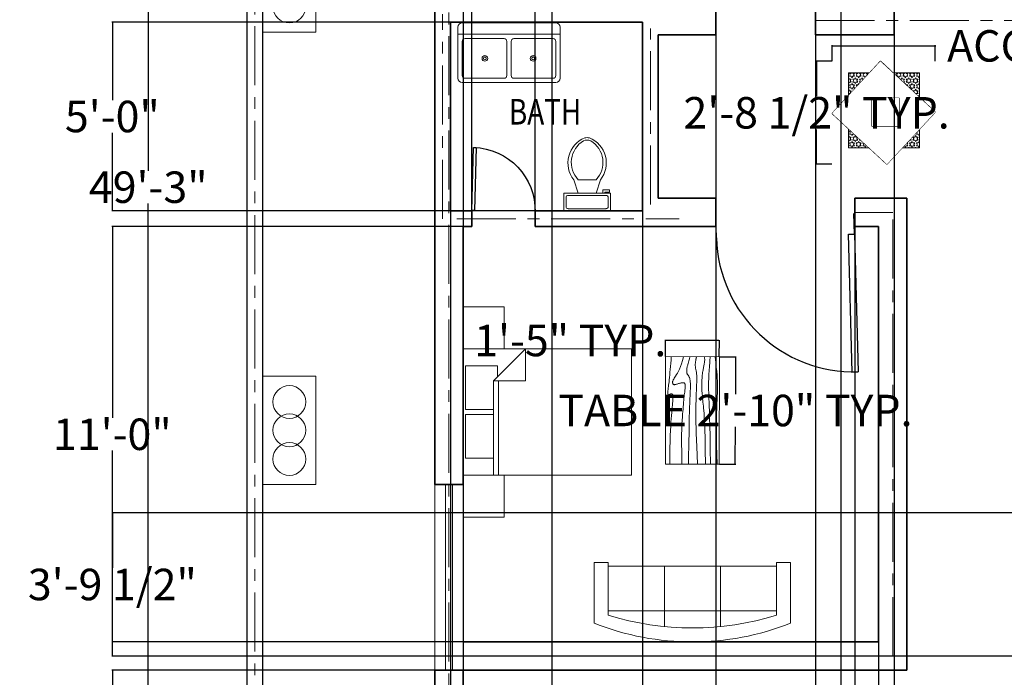
# Model space of a CAD drawing. Units: inches. Extents: x 541 to 1172, y -20 to 887.
# Tile 3 of 8: x 544 to 857, y 378 to 587. Entities that reach past the tile are written whole.
import ezdxf

# ---------------------------------------------------------------- set-up
doc = ezdxf.new("R2010")
doc.units = ezdxf.units.IN
doc.header["$MEASUREMENT"] = 0
doc.set_wipeout_variables(frame=1)
doc.linetypes.add('CENTER', pattern=[50.8, 31.75, -6.35, 6.35, -6.35])
doc.layers.get('0').update_dxf_attribs({"color": 70})
for name, color, linetype, lineweight in [('A-ANNO-DIMS', 2, 'Continuous', 18), ('A-AREA-IDEN', 7, 'Continuous', 20), ('A-DOOR', 4, 'Continuous', 25), ('A-FLOR-FIXT', 9, 'Continuous', 18), ('A-FURN', 30, 'Continuous', 18), ('A-WALL-CNTR', 1, 'CENTER', 13), ('L-PLNT', 70, 'Continuous', 18), ('L-SITE-WALL', 7, 'Continuous', 30), ('WALL', 7, 'Continuous', 35), ('WINDOW', 2, 'Continuous', 18)]:
    doc.layers.add(name, color=color, linetype=linetype, lineweight=lineweight)
doc.styles.get("Standard").update_dxf_attribs({"font": 'arial.ttf'})
doc.styles.add('YQ_DIM', font='SUPEROS.SHX', dxfattribs={"width": 0.8, "bigfont": 'HZDX.SHX'})
doc.dimstyles.get("Standard").update_dxf_attribs({"dimtxt": 10, "dimasz": 0.18, "dimexe": 0.18, "dimexo": 0.0625, "dimgap": 0.09, "dimtad": 0, "dimtih": 1, "dimtoh": 1, "dimdec": 1, "dimzin": 0, "dimdsep": 46, "dimlunit": 4, "dimtxsty": 'Standard', "dimcen": 0.09, "dimadec": 0, "dimazin": 0, "dimtfac": 1, "dimtdec": 1, "dimtofl": 0, "dimtmove": 0, "dimatfit": 3, "dimfxl": 1, "dimtolj": 1, "dimtzin": 0, "dimarcsym": 0})

# ---------------------------------------------------------------- blocks, each defined once
blk = doc.blocks.new('*D3')
at = {"layer": 'A-ANNO-DIMS', "color": 0, "lineweight": -2, "transparency": 16777216}
for p, q in [((616.57, 829.68), (585.07, 829.68)), ((585.25, 829.5), (585.25, 539.38)), ((585.25, 238.86), (585.25, 528.98)), ((621.57, 238.68), (585.07, 238.68))]:
    blk.add_line(p, q, dxfattribs=at)
for points in [[(585.22, 829.5), (585.28, 829.5), (585.25, 829.68)], [(585.22, 238.86), (585.28, 238.86), (585.25, 238.68)]]:
    blk.add_solid(points, dxfattribs=at)
at = {"layer": 'Defpoints', "color": 0, "lineweight": -2, "transparency": 16777216}
for p in [(616.64, 829.68), (585.25, 238.68), (621.64, 238.68)]:
    blk.add_point(p, dxfattribs=at)
at = {"layer": 'A-ANNO-DIMS', "color": 0, "transparency": 16777216, "insert": (585.25, 534.18), "char_height": 10, "attachment_point": 5}
blk.add_mtext('\\A1;49\'-3"', dxfattribs=at)
blk = doc.blocks.new('Bed - Queen')
for p, q in [((0, -80.00003), (0, 0)), ((0, 0), (59.99999, 0)), ((59.99999, 0), (59.99999, -80.00003)), ((7.99999, -1.2), (28.79998, -1.2)), ((7.99999, -14.4), (7.99999, -1.2)), ((28.79998, -1.2), (28.79998, -14.4)), ((31.19999, -1.2), (51.99999, -1.2)), ((31.19999, -14.4), (31.19999, -1.2)), ((51.99999, -1.2), (51.99999, -16.4)), ((0, -14.4), (44.8, -14.4)), ((44.8, -16.8), (0, -16.8)), ((59.99999, -29.6), (44.8, -14.4)), ((44.8, -14.4), (44.8, -29.6)), ((51.99999, -16.4), (46.79936, -16.4)), ((44.8, -29.6), (59.99999, -29.6)), ((59.99999, -80.00003), (0, -80.00003))]:
    blk.add_line(p, q)
blk = doc.blocks.new('Table - Rectangular Woodgrain 60 x 30 in.')
for p, q in [((0, 0), (0, -30)), ((60, 0), (0, 0)), ((60, -30), (60, 0)), ((0, -30), (60, -30))]:
    blk.add_line(p, q)
for points in [[(0, -2.4), (4.8155, -2.418), (9.0302, -2.4688), (12.709, -2.5477), (15.9167, -2.65), (18.7181, -2.7711), (21.1781, -2.9063), (23.3616, -3.0508), (25.3333, -3.2), (27.1477, -3.3495), (28.8172, -3.4958), (30.3437, -3.636), (31.7291, -3.7667), (32.9756, -3.8849), (34.0849, -3.9875), (35.059, -4.0714), (35.9, -4.1334), (36.6114, -4.1711), (37.2041, -4.1854), (37.6906, -4.1779), (38.0833, -4.15), (38.3948, -4.1034), (38.6375, -4.0396), (38.8239, -3.9602), (38.9666, -3.8667), (39.0764, -3.7608), (39.1573, -3.6448), (39.2116, -3.521), (39.2416, -3.3917), (39.2498, -3.2593), (39.2385, -3.1261), (39.21, -2.9944), (39.1666, -2.8667), (39.111, -2.7447), (39.0468, -2.6281), (38.978, -2.5163), (38.9083, -2.4083), (38.8418, -2.3035), (38.7823, -2.201), (38.7337, -2.1001), (38.7, -2), (38.6844, -1.9003), (38.6875, -1.8021), (38.7094, -1.707), (38.75, -1.6167), (38.8094, -1.5326), (38.8875, -1.4563), (38.9844, -1.3893), (39.1, -1.3333), (39.2351, -1.2896), (39.3937, -1.2583), (39.5804, -1.2396), (39.8, -1.2333), (40.057, -1.2396), (40.3562, -1.2583), (40.7023, -1.2896), (41.1, -1.3333), (41.5547, -1.3895), (42.0755, -1.4573), (42.6721, -1.5361), (43.3542, -1.625), (44.1316, -1.7233), (45.014, -1.8302), (46.0114, -1.9449), (47.1333, -2.0667), (48.3862, -2.1947), (49.7625, -2.3281), (51.2513, -2.4663), (52.8416, -2.6083), (54.5226, -2.7535), (56.2833, -2.9011), (58.1127, -3.0501), (60, -3.2)], [(0, -9.2), (6.5759, -9.0858), (11.9385, -9.0365), (16.2527, -9.0418), (19.6833, -9.0917), (22.3952, -9.1759), (24.5531, -9.2844), (26.322, -9.4069), (27.8666, -9.5333), (29.3241, -9.6553), (30.7203, -9.7719), (32.0532, -9.8837), (33.3208, -9.9917), (34.5213, -10.0965), (35.6526, -10.199), (36.7128, -10.2999), (37.7, -10.4), (38.6129, -10.4996), (39.4531, -10.5969), (40.223, -10.6895), (40.925, -10.775), (41.5613, -10.8512), (42.1344, -10.9156), (42.6465, -10.966), (43.1, -11), (43.4976, -11.0158), (43.8437, -11.0136), (44.143, -10.9942), (44.4, -10.9583), (44.6195, -10.9069), (44.8062, -10.8406), (44.9648, -10.7603), (45.1, -10.6667), (45.2155, -10.5598), (45.3114, -10.4365), (45.3871, -10.2929), (45.4416, -10.125), (45.4743, -9.929), (45.4844, -9.7011), (45.4709, -9.4371), (45.4333, -9.1333), (45.3716, -8.7883), (45.2896, -8.4104), (45.1919, -8.0107), (45.0833, -7.6), (44.9685, -7.1893), (44.8521, -6.7896), (44.7388, -6.4117), (44.6333, -6.0667), (44.54, -5.7628), (44.4614, -5.4979), (44.4001, -5.2675), (44.3583, -5.0667), (44.3384, -4.8909), (44.3427, -4.7354), (44.3736, -4.5956), (44.4333, -4.4667), (44.5236, -4.3453), (44.6427, -4.2333), (44.7884, -4.1339), (44.9583, -4.05), (45.1501, -3.9849), (45.3614, -3.9417), (45.59, -3.9234), (45.8333, -3.9333), (46.0915, -3.9749), (46.3734, -4.0531), (46.6906, -4.1736), (47.0542, -4.3417), (47.4756, -4.5629), (47.9661, -4.8427), (48.5372, -5.1866), (49.2, -5.6), (49.9676, -6.0844), (50.8594, -6.625), (51.8965, -7.2031), (53.1, -7.8), (54.491, -8.3969), (56.0906, -8.975), (57.9199, -9.5156), (60, -10)], [(0, -12.8), (5.1847, -12.9322), (9.6213, -13.0323), (13.3963, -13.1059), (16.5958, -13.1583), (19.3063, -13.1952), (21.614, -13.2219), (23.6054, -13.2439), (25.3666, -13.2667), (26.9728, -13.2947), (28.4531, -13.3281), (29.8256, -13.3663), (31.1083, -13.4083), (32.3191, -13.4535), (33.476, -13.501), (34.597, -13.5501), (35.7, -13.6), (36.7984, -13.6497), (37.8875, -13.6979), (38.9578, -13.743), (40, -13.7833), (41.0047, -13.8174), (41.9625, -13.8438), (42.864, -13.8607), (43.7, -13.8667), (44.4631, -13.8604), (45.1552, -13.8417), (45.7801, -13.8104), (46.3416, -13.7667), (46.8439, -13.7104), (47.2906, -13.6417), (47.6858, -13.5604), (48.0333, -13.4667), (48.3375, -13.3608), (48.6042, -13.2448), (48.8396, -13.121), (49.05, -12.9917), (49.2417, -12.8593), (49.4208, -12.7261), (49.5937, -12.5944), (49.7667, -12.4667), (49.9452, -12.3451), (50.1323, -12.2313), (50.3303, -12.1268), (50.5416, -12.0333), (50.7686, -11.9524), (51.0135, -11.8854), (51.2788, -11.8341), (51.5666, -11.8), (51.8785, -11.7843), (52.2116, -11.7865), (52.562, -11.8059), (52.926, -11.8417), (53.2998, -11.8931), (53.6795, -11.9594), (54.0614, -12.0397), (54.4416, -12.1333), (54.8223, -12.2401), (55.2293, -12.3625), (55.6942, -12.5037), (56.2489, -12.6667), (56.9251, -12.8547), (57.7545, -13.0708), (58.7689, -13.3182), (60, -13.6)], [(0, -18), (5.124, -17.7273), (9.6609, -17.5057), (13.6705, -17.3303), (17.2125, -17.1958), (20.3467, -17.0973), (23.1328, -17.0297), (25.6307, -16.9878), (27.9, -16.9667), (29.9928, -16.9617), (31.9302, -16.9703), (33.7254, -16.9907), (35.3917, -17.0208), (36.9423, -17.0588), (38.3906, -17.1026), (39.7499, -17.1503), (41.0333, -17.2), (42.2519, -17.2496), (43.4073, -17.2969), (44.4986, -17.3395), (45.525, -17.375), (46.4858, -17.4012), (47.3802, -17.4156), (48.2074, -17.416), (48.9667, -17.4), (49.6583, -17.3662), (50.2872, -17.3167), (50.8595, -17.2547), (51.3812, -17.1833), (51.8584, -17.1057), (52.2971, -17.025), (52.7034, -16.9443), (53.0833, -16.8667), (53.443, -16.7951), (53.789, -16.7313), (54.128, -16.6768), (54.4666, -16.6334), (54.8115, -16.6024), (55.1693, -16.5854), (55.5465, -16.5841), (55.95, -16.6), (56.3828, -16.6337), (56.8346, -16.6823), (57.2915, -16.7418), (57.7396, -16.8084), (58.165, -16.878), (58.5539, -16.9469), (58.8924, -17.0111), (59.1666, -17.0667), (59.3679, -17.1107), (59.5078, -17.1438), (59.6032, -17.1675), (59.6708, -17.1833), (59.7275, -17.193), (59.7901, -17.1979), (59.8753, -17.1998), (60, -17.2)], [(0, -22.4), (8.0098, -22.2501), (14.4094, -22.1011), (19.4168, -21.9535), (23.25, -21.8083), (26.1269, -21.6663), (28.2656, -21.5281), (29.884, -21.3947), (31.2, -21.2667), (32.3967, -21.1448), (33.5172, -21.0292), (34.5697, -20.9198), (35.5625, -20.8167), (36.5037, -20.7198), (37.4015, -20.6292), (38.2642, -20.5448), (39.1, -20.4667), (39.9164, -20.3951), (40.7187, -20.3313), (41.5117, -20.2768), (42.3, -20.2333), (43.0883, -20.2024), (43.8812, -20.1854), (44.6836, -20.1841), (45.5, -20.2), (46.3328, -20.234), (47.1747, -20.2844), (48.0163, -20.3488), (48.8479, -20.425), (49.66, -20.5106), (50.4429, -20.6031), (51.1872, -20.7004), (51.8833, -20.8), (52.5246, -20.8999), (53.1166, -20.9995), (53.6681, -21.0983), (54.1875, -21.1958), (54.6834, -21.2919), (55.1646, -21.3859), (55.6394, -21.4777), (56.1167, -21.5667), (56.6028, -21.6515), (57.0961, -21.7266), (57.5929, -21.7852), (58.0896, -21.8208), (58.5823, -21.8268), (59.0674, -21.7964), (59.5412, -21.723), (60, -21.6)], [(0, -25.2), (8.6355, -25.0504), (15.7026, -24.9031), (21.4049, -24.7606), (25.9458, -24.625), (29.529, -24.4988), (32.3578, -24.3844), (34.6359, -24.284), (36.5667, -24.2), (38.3213, -24.1341), (39.9417, -24.0854), (41.437, -24.0523), (42.8167, -24.0333), (44.0901, -24.0268), (45.2667, -24.0313), (46.3557, -24.0451), (47.3667, -24.0667), (48.309, -24.0947), (49.1928, -24.1287), (50.0284, -24.168), (50.826, -24.2125), (51.5959, -24.2617), (52.3483, -24.3151), (53.0935, -24.3725), (53.8417, -24.4334), (54.6009, -24.497), (55.3699, -24.561), (56.1454, -24.6226), (56.9239, -24.6792), (57.7021, -24.7279), (58.4764, -24.7662), (59.2435, -24.7911), (60, -24.8)], [(0, -28.8), (5.6867, -28.6681), (10.45, -28.5698), (14.407, -28.5012), (17.675, -28.4584), (20.3711, -28.4374), (22.6125, -28.4344), (24.5164, -28.4455), (26.2, -28.4667), (27.762, -28.4947), (29.2276, -28.5281), (30.6033, -28.5663), (31.8958, -28.6084), (33.1118, -28.6535), (34.2578, -28.7011), (35.3405, -28.7501), (36.3666, -28.8), (37.3443, -28.8497), (38.288, -28.8974), (39.2137, -28.9412), (40.1375, -28.9792), (41.0753, -29.0093), (42.0432, -29.0297), (43.0572, -29.0384), (44.1333, -29.0333), (45.2936, -29.0114), (46.5843, -28.9641), (48.0579, -28.8816), (49.7666, -28.7542), (51.7629, -28.5721), (54.0989, -28.3255), (56.8272, -28.0048), (60, -27.6)]]:
    blk.add_lwpolyline(points)
blk = doc.blocks.new('Sofa - Roundback 7 ft.')
for p, q in [((-12.00002, -32.4421), (-12.00003, -6.5971)), ((11.99997, -32.4421), (11.99998, -6.5971)), ((-36.000027, -34), (-36.000027, -11.4696)), ((35.99998, -34), (35.99998, -11.4696)), ((-35.999844, -13.3819), (35.9998, -13.3819)), ((-36.000027, -32.4421), (35.99998, -32.4421))]:
    blk.add_line(p, q)
for points in [[(-36.000027, -34), (-42.000027, -34), (-42.000027, -8)], [(41.99998, -8), (41.99998, -34), (35.99998, -34)]]:
    blk.add_lwpolyline(points)
for centre, radius, start, end in [((0, -114.25), 114.25, 68.43141, 111.5686), ((-0.00001, -127.1968), 121.1968, 72.72033, 107.2797)]:
    blk.add_arc(centre, radius, start, end)
blk = doc.blocks.new('*U23')
for p, q in [((0, 0), (0, -6)), ((40, 0), (40, -6))]:
    blk.add_line(p, q)
blk.add_lwpolyline([(0, 0), (0, 40), (1.75, 40), (1.75, 0)], close=True)
blk.add_arc((0, 0), 40, 0, 90)
blk = doc.blocks.new('*U28')
for p, q in [((9.5, -6), (9.5, -2)), ((-10, -8.5), (-8, -8.5)), ((-10, -9.5), (-10, -8.5)), ((-8, -8.5), (-8, -8)), ((-7, -8), (-7, -9.5)), ((-4, -8), (-6, -14)), ((4, -8), (6, -14)), ((-7, -9.5), (-10, -9.5)), ((4, -14), (-4, -14))]:
    blk.add_line(p, q)
blk.add_lwpolyline([(10.5, -8), (10.5, 0), (-10.5, 0), (-10.5, -8)], close=True)
for points in [[(-9.5, -2), (-9.5, -6)], [(8.5, -1), (-8.5, -1)], [(-8.5, -7), (8.5, -7)]]:
    blk.add_lwpolyline(points)
for centre, radius, start, end in [((-8.62, -1.88), 0.884, 81.8699, 188.1301), ((8.62, -1.88), 0.884, 351.8699, 98.1301), ((-8.62, -6.12), 0.884, 171.8699, 278.1301), ((8.62, -6.12), 0.884, 261.8699, 8.1301), ((3.52, -21.58), 12.17, 141.4691, 247.9714), ((4.2, -21.82), 11.33, 136.3677, 238.9468), ((-3.52, -21.58), 12.17, 292.0284, 38.5307), ((-4.2, -21.82), 11.33, 301.053, 43.6321), ((0, -27.88), 4, 245.7318, 294.2682), ((0, -29), 4, 254.8605, 285.1395)]:
    blk.add_arc(centre, radius, start, end)
blk = doc.blocks.new('Sink-double - 36 in top')
for p, q in [((-18, -4), (18, -4)), ((-0.75, -18.5), (-0.75, -6.5)), ((0.75, -6.5), (0.75, -18.5))]:
    blk.add_line(p, q)
for points in [[(-16.5, 0), (16.5, 0)], [(-18, -19.5), (-18, -1.5)], [(18, -1.5), (18, -19.5)], [(-16.5, -18.5), (-16.5, -6.5)], [(-15.5, -5.5), (-1.75, -5.5)], [(1.75, -5.5), (15.5, -5.5)], [(16.5, -6.5), (16.5, -18.5)], [(-1.75, -19.5), (-15.5, -19.5)], [(15.5, -19.5), (1.75, -19.5)], [(16.5, -21), (-16.5, -21)]]:
    blk.add_lwpolyline(points)
for centre, radius in [((-8.5, -12.5), 1), ((-8.5, -12.5), 0.5), ((8.5, -12.5), 1), ((8.5, -12.5), 0.5)]:
    blk.add_circle(centre, radius)
for centre, radius, start, end in [((-16.5, -1.5), 1.5, 90, 180), ((16.5, -1.5), 1.5, 0, 90), ((-15.5, -6.5), 1, 90, 180), ((-1.75, -6.5), 1, 0, 90), ((1.75, -6.5), 1, 90, 180), ((15.5, -6.5), 1, 0, 90), ((-16.5, -19.5), 1.5, 180, 270), ((-15.5, -18.5), 1, 180, 270), ((-1.75, -18.5), 1, 270, 0), ((1.75, -18.5), 1, 180, 270), ((15.5, -18.5), 1, 270, 0), ((16.5, -19.5), 1.5, 270, 0)]:
    blk.add_arc(centre, radius, start, end)
blk = doc.blocks.new('*U29')
for p, q in [((0, 0), (0, -6)), ((-40, 0), (-40, -6))]:
    blk.add_line(p, q)
blk.add_lwpolyline([(0, 0), (0, 40), (-1.75, 40), (-1.75, 0)], close=True)
blk.add_arc((0, 0), 40, 90, 180)
blk = doc.blocks.new('WD_WIN4')
at = {"lineweight": -2}
for p, q in [((-0.5, 0.5), (0.5, 0.5)), ((-0.5, 0.12), (0.5, 0.12)), ((-0.5, -0.12), (0.5, -0.12)), ((-0.5, -0.5), (0.5, -0.5))]:
    blk.add_line(p, q, dxfattribs=at)
blk = doc.blocks.new('PLANTER-THREE-ROUND')
blk.add_lwpolyline([(34.49, 16.89), (0, 16.89), (0, 0), (34.49, 0)], close=True)
for centre in [(8.25, 8.45), (17.25, 8.45), (26.39, 8.45)]:
    blk.add_circle(centre, 5.21)
blk = doc.blocks.new('FURN-ACCENT-SQUARE')
h = blk.add_hatch()
h.set_pattern_fill('STARS', color=256, scale=4.255607)
h.set_pattern_definition([(0, (-199.5324, -51.5532), (0, 0.921366), [0.531951, -0.531951]), (60, (-199.5324, -51.5532), (-0.7979263, 0.460683), [0.531951, -0.531951]), (120, (-199.2664, -51.0925), (-0.7979263, -0.460683), [0.531951, -0.531951])])
h.paths.add_polyline_path([(27.75, 29.01), (5.18, 29.01), (5.18, 5.24), (27.75, 5.24)])
for points in [[(0, 16.17), (15.35, 32.72), (32.78, 16.55), (17.43, 0)], [(5.18, 29.01), (27.75, 29.01), (27.75, 5.24), (5.18, 5.24)]]:
    blk.add_lwpolyline(points, close=True)
blk.add_wipeout([(32.78, 16.55), (17.43, 0), (0, 16.17), (15.35, 32.72)])
blk.add_lwpolyline([(12.67, 21.04), (21.3, 21.04), (21.3, 12.15), (12.67, 12.15)], close=True)
blk.add_wipeout([(21.3, 12.15), (12.67, 12.15), (12.67, 21.04), (21.3, 21.04), (21.3, 21.04)])
blk = doc.blocks.new('FURN-NIGHTSTAND')
for p, q in [((0, 13.4), (0, 0)), ((0, 0), (13, 0))]:
    blk.add_line(p, q)
blk = doc.blocks.new('*D57')
at = {"layer": 'A-ANNO-DIMS', "color": 0, "lineweight": -2, "transparency": 16777216}
for p, q in [((766.74, 480.3), (771.98, 480.29)), ((771.8, 480.11), (771.78, 468.4)), ((771.74, 446.31), (771.76, 458.01)), ((766.68, 446.13), (771.92, 446.13))]:
    blk.add_line(p, q, dxfattribs=at)
for points in [[(771.77, 480.11), (771.83, 480.11), (771.8, 480.29)], [(771.71, 446.31), (771.77, 446.31), (771.74, 446.13)]]:
    blk.add_solid(points, dxfattribs=at)
at = {"layer": 'Defpoints', "color": 0, "lineweight": -2, "transparency": 16777216}
for p in [(766.67, 480.3), (771.8, 480.29), (766.62, 446.13)]:
    blk.add_point(p, dxfattribs=at)
at = {"layer": 'A-ANNO-DIMS', "color": 0, "transparency": 16777216, "insert": (771.77, 463.21), "char_height": 10, "attachment_point": 5}
blk.add_mtext('\\A1;TABLE 2\'-10" TYP.', dxfattribs=at)
blk = doc.blocks.new('*D58')
at = {"layer": 'A-ANNO-DIMS', "color": 0, "lineweight": -2, "transparency": 16777216}
for p, q in [((749.6, 485.45), (749.42, 485.45)), ((749.59, 480.39), (749.6, 485.63)), ((766.5, 485.42), (749.78, 485.45)), ((766.67, 480.36), (766.68, 485.6))]:
    blk.add_line(p, q, dxfattribs=at)
for points in [[(749.78, 485.48), (749.78, 485.42), (749.6, 485.45)], [(766.5, 485.45), (766.5, 485.39), (766.68, 485.42)]]:
    blk.add_solid(points, dxfattribs=at)
at = {"layer": 'Defpoints', "color": 0, "lineweight": -2, "transparency": 16777216}
for p in [(749.6, 485.45), (749.59, 480.33), (766.67, 480.3)]:
    blk.add_point(p, dxfattribs=at)
at = {"layer": 'A-ANNO-DIMS', "color": 0, "transparency": 16777216, "insert": (719.32, 485.45), "char_height": 10, "attachment_point": 5}
blk.add_mtext('\\A1;1\'-5" TYP.', dxfattribs=at)
blk = doc.blocks.new('*D61')
at = {"layer": 'A-ANNO-DIMS', "color": 0, "lineweight": -2, "transparency": 16777216}
for p, q in [((802.49, 574.25), (802.49, 579.28)), ((802.67, 579.1), (835.09, 579.1)), ((835.27, 574.25), (835.27, 579.28)), ((835.27, 579.1), (835.45, 579.1))]:
    blk.add_line(p, q, dxfattribs=at)
for points in [[(802.67, 579.13), (802.67, 579.07), (802.49, 579.1)], [(835.09, 579.13), (835.09, 579.07), (835.27, 579.1)]]:
    blk.add_solid(points, dxfattribs=at)
at = {"layer": 'Defpoints', "color": 0, "lineweight": -2, "transparency": 16777216}
for p in [(835.27, 579.1), (802.49, 574.19), (835.27, 574.19)]:
    blk.add_point(p, dxfattribs=at)
at = {"layer": 'A-ANNO-DIMS', "color": 0, "transparency": 16777216, "insert": (896.96, 579.1), "char_height": 10, "attachment_point": 5}
blk.add_mtext('\\A1;ACCENT 2\'-9" TYP.', dxfattribs=at)
blk = doc.blocks.new('*D62')
at = {"layer": 'A-ANNO-DIMS', "color": 0, "lineweight": -2, "transparency": 16777216}
for p, q in [((802.42, 574.19), (797.39, 574.19)), ((797.57, 574.01), (797.57, 563.09)), ((797.57, 541.65), (797.57, 552.57)), ((802.42, 541.47), (797.39, 541.47))]:
    blk.add_line(p, q, dxfattribs=at)
for points in [[(797.54, 574.01), (797.6, 574.01), (797.57, 574.19)], [(797.54, 541.65), (797.6, 541.65), (797.57, 541.47)]]:
    blk.add_solid(points, dxfattribs=at)
at = {"layer": 'Defpoints', "color": 0, "lineweight": -2, "transparency": 16777216}
for p in [(797.57, 574.19), (802.49, 574.19), (802.49, 541.47)]:
    blk.add_point(p, dxfattribs=at)
at = {"layer": 'A-ANNO-DIMS', "color": 0, "transparency": 16777216, "insert": (797.57, 557.83), "char_height": 10, "attachment_point": 5}
blk.add_mtext('\\A1;2\'-8 1/2" TYP.', dxfattribs=at)
blk = doc.blocks.new('*D82')
at = {"layer": 'A-ANNO-DIMS', "color": 0, "lineweight": -2, "transparency": 16777216}
for p, q in [((681.28, 586.59), (681.28, -5.37)), ((742.28, 526.59), (742.28, -5.37)), ((681.46, -5.19), (698.4, -5.19)), ((742.1, -5.19), (725.16, -5.19))]:
    blk.add_line(p, q, dxfattribs=at)
for points in [[(681.46, -5.16), (681.46, -5.22), (681.28, -5.19)], [(742.1, -5.16), (742.1, -5.22), (742.28, -5.19)]]:
    blk.add_solid(points, dxfattribs=at)
at = {"layer": 'Defpoints', "color": 0, "lineweight": -2, "transparency": 16777216}
for p in [(681.28, 586.65), (742.28, 526.65), (742.28, -5.19)]:
    blk.add_point(p, dxfattribs=at)
at = {"layer": 'A-ANNO-DIMS', "color": 0, "transparency": 16777216, "insert": (711.78, -5.19), "char_height": 10, "attachment_point": 5}
blk.add_mtext('\\A1;5\'-1"', dxfattribs=at)
blk = doc.blocks.new('*D83')
at = {"layer": 'A-ANNO-DIMS', "color": 0, "lineweight": -2, "transparency": 16777216}
for p, q in [((681.22, 586.65), (573.66, 586.65)), ((573.84, 586.47), (573.84, 561.85)), ((573.84, 526.83), (573.84, 551.46)), ((742.22, 526.65), (573.66, 526.65))]:
    blk.add_line(p, q, dxfattribs=at)
for points in [[(573.81, 586.47), (573.87, 586.47), (573.84, 586.65)], [(573.81, 526.83), (573.87, 526.83), (573.84, 526.65)]]:
    blk.add_solid(points, dxfattribs=at)
at = {"layer": 'Defpoints', "color": 0, "lineweight": -2, "transparency": 16777216}
for p in [(681.28, 586.65), (573.84, 526.65), (742.28, 526.65)]:
    blk.add_point(p, dxfattribs=at)
at = {"layer": 'A-ANNO-DIMS', "color": 0, "transparency": 16777216, "insert": (573.84, 556.65), "char_height": 10, "attachment_point": 5}
blk.add_mtext('\\A1;5\'-0"', dxfattribs=at)
blk = doc.blocks.new('*D84')
at = {"layer": 'A-ANNO-DIMS', "color": 0, "lineweight": -2, "transparency": 16777216}
for p, q in [((685.28, 389.59), (685.28, -5.37)), ((817.28, 389.59), (817.28, -5.37)), ((685.46, -5.19), (734.49, -5.19)), ((817.1, -5.19), (768.08, -5.19))]:
    blk.add_line(p, q, dxfattribs=at)
for points in [[(685.46, -5.16), (685.46, -5.22), (685.28, -5.19)], [(817.1, -5.16), (817.1, -5.22), (817.28, -5.19)]]:
    blk.add_solid(points, dxfattribs=at)
at = {"layer": 'Defpoints', "color": 0, "lineweight": -2, "transparency": 16777216}
for p in [(685.28, 389.65), (817.28, 389.65), (817.28, -5.19)]:
    blk.add_point(p, dxfattribs=at)
at = {"layer": 'A-ANNO-DIMS', "color": 0, "transparency": 16777216, "insert": (751.28, -5.19), "char_height": 10, "attachment_point": 5}
blk.add_mtext('\\A1;11\'-0"', dxfattribs=at)
blk = doc.blocks.new('*D85')
at = {"layer": 'A-ANNO-DIMS', "color": 0, "lineweight": -2, "transparency": 16777216}
for p, q in [((685.22, 521.65), (573.66, 521.65)), ((573.84, 521.47), (573.84, 460.85)), ((573.84, 389.83), (573.84, 450.46)), ((685.22, 389.65), (573.66, 389.65))]:
    blk.add_line(p, q, dxfattribs=at)
for points in [[(573.81, 521.47), (573.87, 521.47), (573.84, 521.65)], [(573.81, 389.83), (573.87, 389.83), (573.84, 389.65)]]:
    blk.add_solid(points, dxfattribs=at)
at = {"layer": 'Defpoints', "color": 0, "lineweight": -2, "transparency": 16777216}
for p in [(573.84, 521.65), (685.28, 521.65), (685.28, 389.65)]:
    blk.add_point(p, dxfattribs=at)
at = {"layer": 'A-ANNO-DIMS', "color": 0, "transparency": 16777216, "insert": (573.84, 455.65), "char_height": 10, "attachment_point": 5}
blk.add_mtext('\\A1;11\'-0"', dxfattribs=at)
blk = doc.blocks.new('*D92')
at = {"layer": 'A-ANNO-DIMS', "color": 0, "lineweight": -2, "transparency": 16777216}
for p, q in [((676.22, 380.65), (573.66, 380.65)), ((573.84, 380.47), (573.84, 310.05)), ((573.84, 229.1), (573.84, 299.53)), ((676.22, 228.92), (573.66, 228.92))]:
    blk.add_line(p, q, dxfattribs=at)
for points in [[(573.81, 380.47), (573.87, 380.47), (573.84, 380.65)], [(573.81, 229.1), (573.87, 229.1), (573.84, 228.92)]]:
    blk.add_solid(points, dxfattribs=at)
at = {"layer": 'Defpoints', "color": 0, "lineweight": -2, "transparency": 16777216}
for p in [(573.84, 380.65), (676.28, 380.65), (676.28, 228.92)]:
    blk.add_point(p, dxfattribs=at)
at = {"layer": 'A-ANNO-DIMS', "color": 0, "transparency": 16777216, "insert": (573.84, 304.79), "char_height": 10, "attachment_point": 5}
blk.add_mtext('\\A1;12\'-7 1/2"', dxfattribs=at)
blk = doc.blocks.new('*D96')
at = {"layer": 'A-ANNO-DIMS', "color": 0, "lineweight": -2, "transparency": 16777216}
for p, q in [((980.22, 430.65), (573.66, 430.65)), ((573.84, 430.47), (573.84, 413.18)), ((573.84, 385.35), (573.84, 402.65)), ((980.22, 385.17), (573.66, 385.17))]:
    blk.add_line(p, q, dxfattribs=at)
for points in [[(573.81, 430.47), (573.87, 430.47), (573.84, 430.65)], [(573.81, 385.35), (573.87, 385.35), (573.84, 385.17)]]:
    blk.add_solid(points, dxfattribs=at)
at = {"layer": 'Defpoints', "color": 0, "lineweight": -2, "transparency": 16777216}
for p in [(573.84, 430.65), (980.28, 430.65), (980.28, 385.17)]:
    blk.add_point(p, dxfattribs=at)
at = {"layer": 'A-ANNO-DIMS', "color": 0, "transparency": 16777216, "insert": (573.84, 407.91), "char_height": 10, "attachment_point": 5}
blk.add_mtext('\\A1;3\'-9 1/2"', dxfattribs=at)
blk = doc.blocks.new('*D99')
at = {"layer": 'A-ANNO-DIMS', "color": 0, "lineweight": -2, "transparency": 16777216}
for p, q in [((765.53, 591.59), (765.53, -5.37)), ((797.19, 591.59), (797.19, -5.37)), ((765.71, -5.19), (797.01, -5.19)), ((797.19, -5.19), (797.37, -5.19))]:
    blk.add_line(p, q, dxfattribs=at)
for points in [[(765.71, -5.16), (765.71, -5.22), (765.53, -5.19)], [(797.01, -5.16), (797.01, -5.22), (797.19, -5.19)]]:
    blk.add_solid(points, dxfattribs=at)
at = {"layer": 'Defpoints', "color": 0, "lineweight": -2, "transparency": 16777216}
for p in [(765.53, 591.65), (797.19, 591.65), (797.19, -5.19)]:
    blk.add_point(p, dxfattribs=at)
at = {"layer": 'A-ANNO-DIMS', "color": 0, "transparency": 16777216, "insert": (822.49, -5.19), "char_height": 10, "attachment_point": 5}
blk.add_mtext('\\A1;2\'-7 1/2"', dxfattribs=at)
blk = doc.blocks.new('*D102')
at = {"layer": 'A-ANNO-DIMS', "color": 0, "lineweight": -2, "transparency": 16777216}
for p, q in [((822.26, 582.59), (822.26, -5.37)), ((866.83, 582.59), (866.83, -5.37)), ((822.44, -5.19), (866.65, -5.19)), ((866.83, -5.19), (867.01, -5.19))]:
    blk.add_line(p, q, dxfattribs=at)
for points in [[(822.44, -5.16), (822.44, -5.22), (822.26, -5.19)], [(866.65, -5.16), (866.65, -5.22), (866.83, -5.19)]]:
    blk.add_solid(points, dxfattribs=at)
at = {"layer": 'Defpoints', "color": 0, "lineweight": -2, "transparency": 16777216}
for p in [(822.26, 582.65), (866.83, 582.65), (866.83, -5.19)]:
    blk.add_point(p, dxfattribs=at)
at = {"layer": 'A-ANNO-DIMS', "color": 0, "transparency": 16777216, "insert": (892.04, -5.19), "char_height": 10, "attachment_point": 5}
blk.add_mtext('\\A1;3\'-8 1/2"', dxfattribs=at)
blk = doc.blocks.new('*D105')
at = {"layer": 'A-ANNO-DIMS', "color": 0, "lineweight": -2, "transparency": 16777216}
for p, q in [((797.19, 591.59), (797.19, -5.37)), ((805.28, 591.59), (805.28, -5.37)), ((797.37, -5.19), (805.1, -5.19)), ((805.28, -5.19), (805.46, -5.19))]:
    blk.add_line(p, q, dxfattribs=at)
for points in [[(797.37, -5.16), (797.37, -5.22), (797.19, -5.19)], [(805.1, -5.16), (805.1, -5.22), (805.28, -5.19)]]:
    blk.add_solid(points, dxfattribs=at)
at = {"layer": 'Defpoints', "color": 0, "lineweight": -2, "transparency": 16777216}
for p in [(797.19, 591.65), (805.28, 591.65), (805.28, -5.19)]:
    blk.add_point(p, dxfattribs=at)
at = {"layer": 'A-ANNO-DIMS', "color": 0, "transparency": 16777216, "insert": (818.84, -5.19), "char_height": 10, "attachment_point": 5}
blk.add_mtext('\\A1;0\'-8"', dxfattribs=at)
blk = doc.blocks.new('*D106')
at = {"layer": 'A-ANNO-DIMS', "color": 0, "lineweight": -2, "transparency": 16777216}
for p, q in [((685.28, 735.59), (685.28, -5.37)), ((713.47, 735.15), (713.47, -5.37)), ((685.46, -5.19), (685.91, -5.19)), ((713.29, -5.19), (712.84, -5.19))]:
    blk.add_line(p, q, dxfattribs=at)
for points in [[(685.46, -5.16), (685.46, -5.22), (685.28, -5.19)], [(713.29, -5.16), (713.29, -5.22), (713.47, -5.19)]]:
    blk.add_solid(points, dxfattribs=at)
at = {"layer": 'Defpoints', "color": 0, "lineweight": -2, "transparency": 16777216}
for p in [(685.28, 735.65), (713.47, 735.22), (685.28, -5.19)]:
    blk.add_point(p, dxfattribs=at)
at = {"layer": 'A-ANNO-DIMS', "color": 0, "transparency": 16777216, "insert": (699.38, -5.19), "char_height": 10, "attachment_point": 5}
blk.add_mtext('\\A1;2\'-4"', dxfattribs=at)
blk = doc.blocks.new('*D108')
at = {"layer": 'A-ANNO-DIMS', "color": 0, "lineweight": -2, "transparency": 16777216}
for p, q in [((765.54, 521.59), (765.54, -5.37)), ((809.68, 521.59), (809.68, -5.37)), ((765.72, -5.19), (774.23, -5.19)), ((809.5, -5.19), (800.99, -5.19))]:
    blk.add_line(p, q, dxfattribs=at)
for points in [[(765.72, -5.16), (765.72, -5.22), (765.54, -5.19)], [(809.5, -5.16), (809.5, -5.22), (809.68, -5.19)]]:
    blk.add_solid(points, dxfattribs=at)
at = {"layer": 'Defpoints', "color": 0, "lineweight": -2, "transparency": 16777216}
for p in [(765.54, 521.65), (809.68, 521.65), (809.68, -5.19)]:
    blk.add_point(p, dxfattribs=at)
at = {"layer": 'A-ANNO-DIMS', "color": 0, "transparency": 16777216, "insert": (787.61, -5.19), "char_height": 10, "attachment_point": 5}
blk.add_mtext('\\A1;3\'-8"', dxfattribs=at)
blk = doc.blocks.new('*D110')
at = {"layer": 'A-ANNO-DIMS', "color": 0, "lineweight": -2, "transparency": 16777216}
for p, q in [((688.04, 521.72), (688.04, 872.66)), ((688.22, 872.48), (707.94, 872.48)), ((708.12, 521.72), (708.12, 872.66)), ((708.12, 872.48), (708.3, 872.48))]:
    blk.add_line(p, q, dxfattribs=at)
for points in [[(688.22, 872.51), (688.22, 872.45), (688.04, 872.48)], [(707.94, 872.51), (707.94, 872.45), (708.12, 872.48)]]:
    blk.add_solid(points, dxfattribs=at)
at = {"layer": 'Defpoints', "color": 0, "lineweight": -2, "transparency": 16777216}
for p in [(708.12, 872.48), (688.04, 521.65), (708.12, 521.65)]:
    blk.add_point(p, dxfattribs=at)
at = {"layer": 'A-ANNO-DIMS', "color": 0, "transparency": 16777216, "insert": (721.21, 872.48), "char_height": 10, "attachment_point": 5}
blk.add_mtext('\\A1;1\'-8"', dxfattribs=at)

msp = doc.modelspace()

# ---------------------------------------------------------------- linework, layer by layer
at = {"layer": 'A-WALL-CNTR', "ltscale": 0.590551}
for p, q in [((619.14, 56.56), (619.14, 827.18)), ((680.78, 233.42), (680.78, 740.15)), ((678.78, 524.15), (678.78, 589.15)), ((797.19, 587.15), (969.78, 587.15)), ((744.78, 528.65), (744.78, 584.65)), ((809.68, 526.15), (821.78, 526.15)), ((821.78, 385.15), (821.78, 526.15)), ((683.28, 524.15), (753.91, 524.15)), ((680.78, 385.15), (821.78, 385.15))]:
    msp.add_line(p, q, dxfattribs=at)
at = {"layer": 'L-SITE-WALL'}
for p, q in [((616.64, 49.68), (616.64, 829.68)), ((621.64, 238.68), (621.64, 824.68))]:
    msp.add_line(p, q, dxfattribs=at)
at = {"layer": 'WALL'}
for p, q in [((676.28, 439.71), (676.28, 744.65)), ((765.53, 582.65), (765.53, 591.65)), ((797.19, 591.65), (797.19, 582.65)), ((822.26, 591.65), (822.26, 582.65)), ((681.28, 526.65), (681.28, 586.65)), ((681.28, 586.65), (742.28, 586.65)), ((742.28, 526.65), (742.28, 586.65)), ((765.53, 582.65), (747.28, 582.65)), ((747.28, 530.65), (747.28, 582.65)), ((797.19, 582.65), (822.26, 582.65)), ((747.28, 530.65), (765.54, 530.65)), ((765.54, 530.65), (765.54, 521.65)), ((809.68, 530.65), (826.28, 530.65)), ((809.68, 521.65), (809.68, 530.65)), ((826.28, 380.65), (826.28, 530.65)), ((681.28, 526.65), (688.04, 526.65)), ((688.04, 526.65), (688.04, 521.65)), ((708.12, 526.21), (708.12, 521.65)), ((708.13, 526.65), (742.28, 526.65)), ((685.28, 521.65), (688.04, 521.65)), ((685.28, 439.71), (685.28, 521.65)), ((708.12, 521.65), (747.28, 521.65)), ((747.28, 521.65), (765.54, 521.65)), ((809.68, 521.65), (817.28, 521.65)), ((817.28, 389.65), (817.28, 521.65)), ((676.28, 439.71), (685.28, 439.71)), ((685.28, 389.65), (817.28, 389.65)), ((676.28, 372.78), (676.28, 380.65)), ((676.28, 380.65), (685.28, 380.65)), ((685.28, 380.65), (826.28, 380.65)), ((685.28, 372.78), (685.28, 380.65))]:
    msp.add_line(p, q, dxfattribs=at)

# ---------------------------------------------------------------- block references
at = {"layer": 'A-DOOR'}
for name, p, xscale, yscale, zscale, rotation in [('*U29', (688.05, 526.75), -0.501980870151212, 0.501980870151212, 0.501980870151212, 358.4510988302025), ('*U23', (809.58, 519.29), 1.096315168512706, 1.096315168512706, 1.096315168512706, 181.5489011697975)]:
    msp.add_blockref(name, p, dxfattribs=dict(at, xscale=xscale, yscale=yscale, zscale=zscale, rotation=rotation))
at = {"layer": 'A-FLOR-FIXT', "xscale": 0.9019743609965102, "yscale": 0.9019743609965102, "zscale": 0.9019743609965102}
msp.add_blockref('Sink-double - 36 in top', (699.86, 586.4), dxfattribs=at)
at = {"layer": 'A-FLOR-FIXT', "xscale": 0.7059824596600022, "yscale": 0.7059824596600022, "zscale": 0.7059824596600022, "rotation": 180.0000000000005}
msp.add_blockref('*U28', (724.67, 526.65), dxfattribs=at)
at = {"layer": 'A-FURN'}
msp.add_blockref('FURN-ACCENT-SQUARE', (802.49, 541.47), dxfattribs=at)
at = {"layer": 'A-FURN', "rotation": 180}
msp.add_blockref('FURN-NIGHTSTAND', (698.29, 496.17), dxfattribs=at)
at = {"layer": 'A-FURN'}
for name, p, xscale, yscale, zscale, rotation in [('Bed - Queen', (685.28, 442.67), 0.6685054037368693, 0.6685054037368693, 0.6685054037368693, 89.99999999999999), ('Table - Rectangular Woodgrain 60 x 30 in.', (749.54, 446.16), 0.5694163205475999, 0.5694163205475999, 0.5694163205475999, 89.90810628648191), ('Sofa - Roundback 7 ft.', (758.12, 389.65), 0.7424226432878923, 0.7424226432878923, 0.7424226432878923, 180)]:
    msp.add_blockref(name, p, dxfattribs=dict(at, xscale=xscale, yscale=yscale, zscale=zscale, rotation=rotation))
at = {"layer": 'A-FURN', "extrusion": (0, 0, -1), "zscale": -1}
msp.add_blockref('FURN-NIGHTSTAND', (-698.29, 429.27), dxfattribs=at)
at = {"layer": 'L-PLNT'}
for p, rotation in [((621.64, 617.98), 269.9999999999998), ((621.64, 474.17), 270.0000000000004)]:
    msp.add_blockref('PLANTER-THREE-ROUND', p, dxfattribs=dict(at, rotation=rotation))
at = {"layer": 'WINDOW', "xscale": 59.05511811023622, "yscale": 8.999999999999318, "zscale": 59.05511811023622, "rotation": 89.99999999999979}
msp.add_blockref('WD_WIN4', (680.78, 410.18), dxfattribs=at)

# ---------------------------------------------------------------- texts
at = {"layer": 'A-AREA-IDEN', "style": 'YQ_DIM', "width": 0.8}
msp.add_text('BATH', height=8.13, dxfattribs=at).set_placement((699.82, 554.1))

# ---------------------------------------------------------------- dimensions: what is measured, and where the dimension line sits
at = {"layer": 'A-ANNO-DIMS'}
for base, p1, p2, picture, middle in [((708.12, 872.48), (688.04, 521.65), (708.12, 521.65), '*D110', (721.21, 872.48)), ((685.28, -5.19), (713.47, 735.22), (685.28, 735.65), '*D106', (699.38, -5.19)), ((742.28, -5.19), (681.28, 586.65), (742.28, 526.65), '*D82', (711.78, -5.19)), ((809.68, -5.19), (765.54, 521.65), (809.68, 521.65), '*D108', (787.61, -5.19)), ((817.28, -5.19), (685.28, 389.65), (817.28, 389.65), '*D84', (751.28, -5.19))]:
    dim = msp.add_linear_dim(base=base, p1=p1, p2=p2, dimstyle='Standard', override={"dimdec": 1, "dimlfac": 1, "dimrnd": 0, "dimzin": 1, "dimdsep": 46, "dimlunit": 4, "dimfrac": 2}, dxfattribs=at)
    dim.commit()
    dim.dimension.update_dxf_attribs({"geometry": picture, "text_midpoint": middle})
for base, p1, p2, override, picture, middle in [((585.25, 238.68), (616.64, 829.68), (621.64, 238.68), {"dimclrd": 0, "dimclre": 0, "dimclrt": 0}, '*D3', (585.25, 534.18)), ((573.84, 526.65), (681.28, 586.65), (742.28, 526.65), {"dimdec": 1, "dimlfac": 1, "dimrnd": 0, "dimzin": 1, "dimdsep": 46, "dimlunit": 4, "dimfrac": 2}, '*D83', (573.84, 556.65)), ((573.84, 521.65), (685.28, 389.65), (685.28, 521.65), {"dimdec": 1, "dimlfac": 1, "dimrnd": 0, "dimzin": 1, "dimdsep": 46, "dimlunit": 4, "dimfrac": 2}, '*D85', (573.84, 455.65)), ((573.84, 430.65), (980.28, 385.17), (980.28, 430.65), {"dimdec": 1, "dimlfac": 1, "dimrnd": 0, "dimzin": 1, "dimdsep": 46, "dimlunit": 4, "dimfrac": 2}, '*D96', (573.84, 407.91)), ((573.84, 380.65), (676.28, 228.92), (676.28, 380.65), {"dimdec": 1, "dimlfac": 1, "dimrnd": 0, "dimzin": 1, "dimdsep": 46, "dimlunit": 4, "dimfrac": 2}, '*D92', (573.84, 304.79))]:
    dim = msp.add_linear_dim(base=base, p1=p1, p2=p2, angle=90, dimstyle='Standard', override=override, dxfattribs=at)
    dim.commit()
    dim.dimension.update_dxf_attribs({"geometry": picture, "text_midpoint": middle})
for base, p1, p2, angle, text, picture, middle in [((749.6, 485.45), (766.67, 480.3), (749.59, 480.33), 179.9081, '<> TYP.', '*D58', (719.32, 485.45)), ((771.8, 480.29), (766.62, 446.13), (766.67, 480.3), 89.9081, 'TABLE <> TYP.', '*D57', (771.77, 463.21))]:
    dim = msp.add_linear_dim(base=base, p1=p1, p2=p2, angle=angle, text=text, dimstyle='Standard', override={"dimdec": 1, "dimlfac": 1, "dimrnd": 0, "dimzin": 1, "dimdsep": 46, "dimlunit": 4, "dimfrac": 2}, dxfattribs=at)
    dim.commit()
    dim.dimension.update_dxf_attribs({"geometry": picture, "text_midpoint": middle})

# ---------------------------------------------------------------- next in the draw order: dimensions: what is measured, and where the dimension line sits
dim = msp.add_linear_dim(base=(835.27, 579.1), p1=(802.49, 574.19), p2=(835.27, 574.19), text='ACCENT <> TYP.', dimstyle='Standard', override={"dimdec": 1, "dimlfac": 1, "dimrnd": 0, "dimzin": 1, "dimdsep": 46, "dimlunit": 4, "dimfrac": 2}, dxfattribs=at)
dim.commit()
dim.dimension.update_dxf_attribs({"geometry": '*D61', "text_midpoint": (896.96, 579.1)})
for base, p1, p2, picture, middle in [((797.19, -5.19), (765.53, 591.65), (797.19, 591.65), '*D99', (822.49, -5.19)), ((805.28, -5.19), (797.19, 591.65), (805.28, 591.65), '*D105', (818.84, -5.19)), ((866.83, -5.19), (822.26, 582.65), (866.83, 582.65), '*D102', (892.04, -5.19))]:
    dim = msp.add_linear_dim(base=base, p1=p1, p2=p2, dimstyle='Standard', override={"dimdec": 1, "dimlfac": 1, "dimrnd": 0, "dimzin": 1, "dimdsep": 46, "dimlunit": 4, "dimfrac": 2}, dxfattribs=at)
    dim.commit()
    dim.dimension.update_dxf_attribs({"geometry": picture, "text_midpoint": middle})
dim = msp.add_linear_dim(base=(797.57, 574.19), p1=(802.49, 541.47), p2=(802.49, 574.19), angle=90, text='<> TYP.', dimstyle='Standard', override={"dimdec": 1, "dimlfac": 1, "dimrnd": 0, "dimzin": 1, "dimdsep": 46, "dimlunit": 4, "dimfrac": 2}, dxfattribs=at)
dim.commit()
dim.dimension.update_dxf_attribs({"geometry": '*D62', "text_midpoint": (797.57, 557.83)})

doc.saveas('drawing.dxf')
